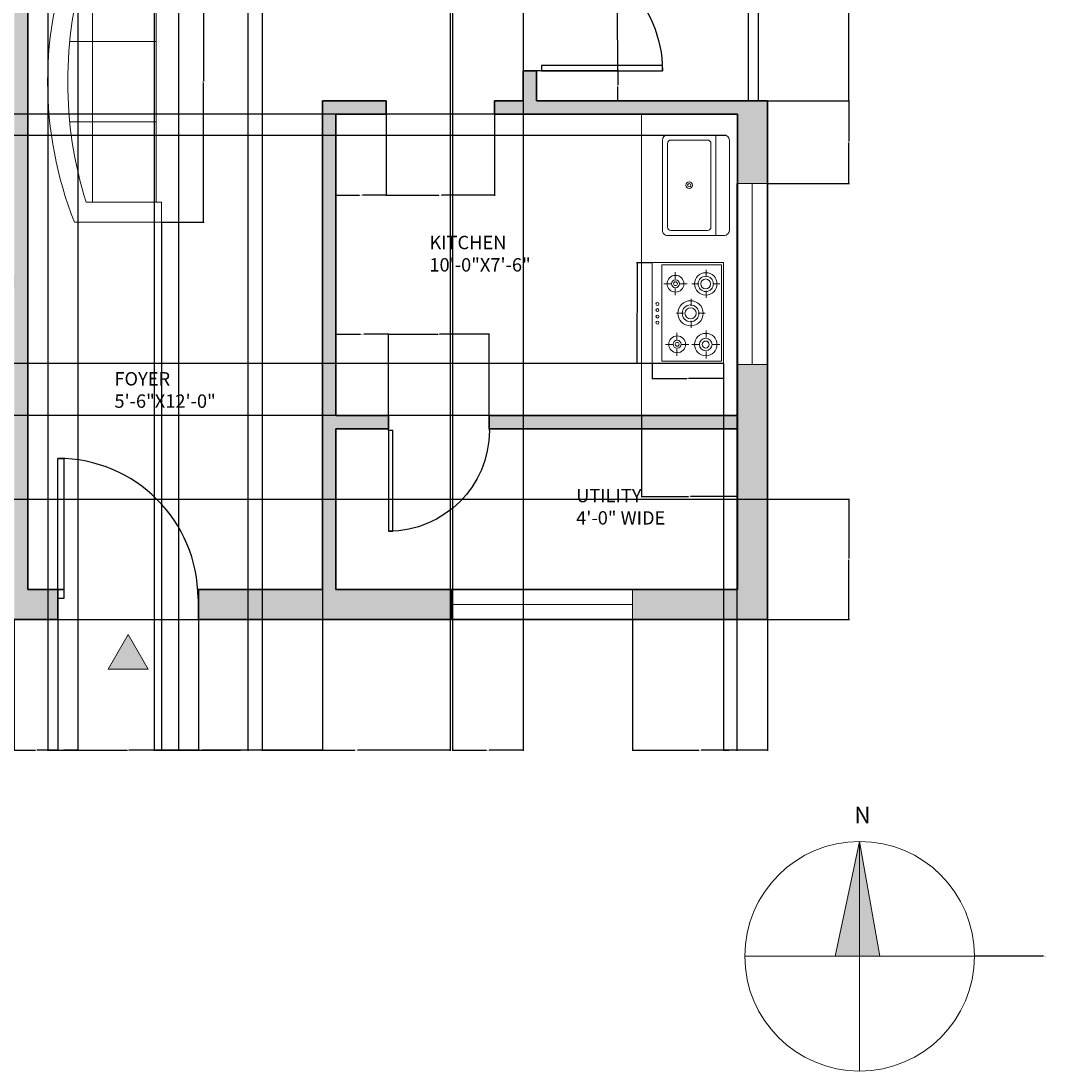
# Model space of a CAD drawing. Units: inches. Extents: x -29 to 443, y -589 to 39.
# Tile 2 of 5: x 136 to 443, y -589 to -275. Entities that reach past the tile are written whole.
import ezdxf

# ---------------------------------------------------------------- set-up
doc = ezdxf.new("R2010")
doc.units = ezdxf.units.IN
for name, color, linetype, lineweight in [('A-ANNO-DIMS', 2, 'Continuous', 18), ('A-ANNO-SYMB', 7, 'Continuous', 18), ('A-AREA-IDEN', 7, 'Continuous', 18), ('A-DOOR', 3, 'Continuous', 25), ('A-EQPM', 8, 'Continuous', 18), ('A-FLOR-CASE', 8, 'Continuous', 18), ('A-FLOR-FIXT', 9, 'Continuous', 18), ('A-FLOR-HRAL', 8, 'Continuous', 25), ('A-FURN', 9, 'Continuous', 18), ('A-GLAZ', 4, 'Continuous', 18), ('A-WALL', 7, 'Continuous', 35)]:
    doc.layers.add(name, color=color, linetype=linetype, lineweight=lineweight)
doc.layers.add('A-WALL-PATT', color=251, linetype='Continuous', lineweight=13, true_color=0x636466)
doc.styles.get("Standard").update_dxf_attribs({"font": 'arial.ttf'})
doc.dimstyles.get("Standard").update_dxf_attribs({"dimtxt": 0.18, "dimasz": 0.18, "dimexe": 0.18, "dimexo": 0.0625, "dimgap": 0.09, "dimtad": 0, "dimtih": 1, "dimtoh": 1, "dimdec": 4, "dimzin": 0, "dimdsep": 46, "dimtxsty": 'Standard', "dimcen": 0.09, "dimadec": 0, "dimazin": 0, "dimtfac": 1, "dimtdec": 4, "dimtofl": 0, "dimtmove": 0, "dimatfit": 3, "dimfxl": 1, "dimtolj": 1, "dimtzin": 0, "dimarcsym": 0})

# ---------------------------------------------------------------- blocks, each defined once
blk = doc.blocks.new('*U3')
for p, q in [((0, 0), (0, -6)), ((40, 0), (40, -6))]:
    blk.add_line(p, q)
blk.add_lwpolyline([(0, 0), (0, 40), (1.75, 40), (1.75, 0)], close=True)
blk.add_arc((0, 0), 40, 0, 90)
blk = doc.blocks.new('Sofa - Roundback 7 ft.')
for p, q in [((-12.00002, -32.4421), (-12.00003, -6.5971)), ((11.99997, -32.4421), (11.99998, -6.5971)), ((-36.000027, -34), (-36.000027, -11.4696)), ((35.99998, -34), (35.99998, -11.4696)), ((-35.999844, -13.3819), (35.9998, -13.3819)), ((-36.000027, -32.4421), (35.99998, -32.4421))]:
    blk.add_line(p, q)
for points in [[(-36.000027, -34), (-42.000027, -34), (-42.000027, -8)], [(41.99998, -8), (41.99998, -34), (35.99998, -34)]]:
    blk.add_lwpolyline(points)
for centre, radius, start, end in [((0, -114.25), 114.25, 68.43141, 111.5686), ((-0.00001, -127.1968), 121.1968, 72.72033, 107.2797)]:
    blk.add_arc(centre, radius, start, end)
blk = doc.blocks.new('Sink-single - 30 in top')
blk.add_line((-15, -3.999996), (15, -3.999996))
for points in [[(-13.5, 0), (13.5, 0)], [(-15, -18.499996), (-15, -1.5)], [(15, -1.5), (15, -18.499996)], [(-12.5, -5.499996), (12.5, -5.499996)], [(-13.5, -17.499996), (-13.5, -6.499996)], [(13.5, -6.499996), (13.5, -17.499996)], [(12.5, -18.499996), (-12.5, -18.499996)], [(13.5, -19.999996), (-13.5, -19.999996)]]:
    blk.add_lwpolyline(points)
for radius in [1, 0.5]:
    blk.add_circle((0, -11.999996), radius)
for centre, radius, start, end in [((-13.5, -1.5), 1.5, 90, 180), ((13.5, -1.5), 1.5, 0, 90), ((-12.5, -6.499996), 1, 90, 180), ((12.5, -6.499996), 1, 0, 90), ((-13.5, -18.499996), 1.5, 180, 270), ((-12.5, -17.499996), 1, 180, 270), ((12.5, -17.499996), 1, 270, 0), ((13.5, -18.499996), 1.5, 270, 0)]:
    blk.add_arc(centre, radius, start, end)
blk = doc.blocks.new('38')
at = {"color": 0}
for p, q in [((4682.26, 13565.85), (4682.26, 13514.85)), ((4754.26, 13565.85), (4682.26, 13565.85)), ((4683.76, 13564.35), (4683.76, 13521.85)), ((4752.76, 13564.35), (4683.76, 13564.35)), ((4697.41, 13558.27), (4697.41, 13563.27)), ((4740.78, 13558.27), (4740.78, 13563.27)), ((4752.76, 13521.85), (4752.76, 13564.35)), ((4754.26, 13514.85), (4754.26, 13565.85)), ((4692.48, 13553.34), (4687.47, 13553.34)), ((4697.41, 13543.15), (4697.41, 13548.16)), ((4707.33, 13553.34), (4702.32, 13553.34)), ((4718.43, 13547.65), (4718.43, 13552.65)), ((4735.85, 13553.34), (4730.84, 13553.34)), ((4740.78, 13543.15), (4740.78, 13548.16)), ((4750.7, 13553.34), (4745.7, 13553.34)), ((4697.4, 13534.82), (4697.4, 13539.82)), ((4713.11, 13542.65), (4708.11, 13542.65)), ((4728.85, 13542.65), (4723.85, 13542.65)), ((4740.72, 13536), (4740.72, 13541.01)), ((4718.43, 13532.28), (4718.43, 13537.28)), ((4737.37, 13532.58), (4732.37, 13532.58)), ((4748.92, 13532.58), (4743.92, 13532.58)), ((4694.05, 13531.4), (4689.04, 13531.4)), ((4697.45, 13523.21), (4697.45, 13528.21)), ((4705.6, 13531.4), (4700.6, 13531.4)), ((4740.78, 13524.39), (4740.78, 13529.4)), ((4683.76, 13521.85), (4752.76, 13521.85)), ((4682.26, 13514.85), (4754.26, 13514.85))]:
    blk.add_line(p, q, dxfattribs=at)
for centre, radius in [((4697.43, 13553.15), 8), ((4697.43, 13553.15), 5.5), ((4697.43, 13553.15), 3.5), ((4740.8, 13553.15), 8), ((4740.8, 13553.15), 4.5), ((4740.8, 13553.15), 2.5), ((4718.49, 13542.29), 9), ((4718.49, 13542.29), 6), ((4718.49, 13542.29), 4), ((4697.32, 13531.51), 6), ((4697.32, 13531.51), 2.85), ((4697.32, 13531.51), 1.35), ((4740.65, 13532.69), 6), ((4740.65, 13532.69), 2.85), ((4740.65, 13532.69), 1.35), ((4711.82, 13518.62), 1.09), ((4716.19, 13518.62), 1.09), ((4720.78, 13518.62), 1.09), ((4725.16, 13518.62), 1.09)]:
    blk.add_circle(centre, radius, dxfattribs=at)
blk = doc.blocks.new('WIN-54IN')
blk.add_line((54, 4.5), (0, 4.5))
blk.add_lwpolyline([(0, 9), (54, 9), (54, 0), (0, 0)], close=True)
blk = doc.blocks.new('*D30')
at = {"layer": 'A-ANNO-DIMS', "color": 0, "lineweight": -2, "transparency": 16777216}
for p, q in [((178.45, -250.92), (191.17, -250.92)), ((190.99, -251.1), (190.99, -292.74)), ((190.99, -334.74), (190.99, -293.11)), ((178.45, -334.92), (191.17, -334.92))]:
    blk.add_line(p, q, dxfattribs=at)
at = {"layer": 'A-ANNO-DIMS', "color": 0, "transparency": 16777216}
for points in [[(190.96, -251.1), (191.02, -251.1), (190.99, -250.92)], [(190.96, -334.74), (191.02, -334.74), (190.99, -334.92)]]:
    blk.add_solid(points, dxfattribs=at)
at = {"layer": 'Defpoints', "color": 0, "transparency": 16777216}
for p in [(178.39, -250.92), (190.99, -250.92), (178.39, -334.92)]:
    blk.add_point(p, dxfattribs=at)
at = {"layer": 'A-ANNO-DIMS', "color": 0, "transparency": 16777216, "insert": (190.99, -292.92), "char_height": 0.18, "attachment_point": 5}
blk.add_mtext('\\A1;SOFA 84', dxfattribs=at)
blk = doc.blocks.new('*D34')
at = {"layer": 'A-ANNO-DIMS', "color": 0, "lineweight": -2, "transparency": 16777216}
for p, q in [((324.89, -346.99), (320.26, -346.99)), ((320.44, -347.17), (320.44, -361.85)), ((320.44, -376.89), (320.44, -362.21)), ((324.89, -377.07), (320.26, -377.07))]:
    blk.add_line(p, q, dxfattribs=at)
at = {"layer": 'A-ANNO-DIMS', "color": 0, "transparency": 16777216}
for points in [[(320.41, -347.17), (320.47, -347.17), (320.44, -346.99)], [(320.41, -376.89), (320.47, -376.89), (320.44, -377.07)]]:
    blk.add_solid(points, dxfattribs=at)
at = {"layer": 'Defpoints', "color": 0, "transparency": 16777216}
for p in [(324.95, -346.99), (320.44, -377.07), (324.95, -377.07)]:
    blk.add_point(p, dxfattribs=at)
at = {"layer": 'A-ANNO-DIMS', "color": 0, "transparency": 16777216, "insert": (320.44, -362.03), "char_height": 0.18, "attachment_point": 5}
blk.add_mtext('\\A1;COOKTOP 30', dxfattribs=at)
blk = doc.blocks.new('*D35')
at = {"layer": 'A-ANNO-DIMS', "color": 0, "lineweight": -2, "transparency": 16777216}
for p, q in [((324.95, -377.13), (324.95, -381.76)), ((346.26, -377.13), (346.26, -381.76)), ((325.13, -381.58), (335.41, -381.58)), ((346.08, -381.58), (335.81, -381.58))]:
    blk.add_line(p, q, dxfattribs=at)
at = {"layer": 'A-ANNO-DIMS', "color": 0, "transparency": 16777216}
for points in [[(325.13, -381.55), (325.13, -381.61), (324.95, -381.58)], [(346.08, -381.55), (346.08, -381.61), (346.26, -381.58)]]:
    blk.add_solid(points, dxfattribs=at)
at = {"layer": 'Defpoints', "color": 0, "transparency": 16777216}
for p in [(324.95, -377.07), (346.26, -377.07), (346.26, -381.58)]:
    blk.add_point(p, dxfattribs=at)
at = {"layer": 'A-ANNO-DIMS', "color": 0, "transparency": 16777216, "insert": (335.61, -381.58), "char_height": 0.18, "attachment_point": 5}
blk.add_mtext('\\A1;21', dxfattribs=at)
blk = doc.blocks.new('*D40')
at = {"layer": 'A-ANNO-DIMS', "color": 0, "lineweight": -2, "transparency": 16777216}
for p, q in [((208.44, 5.32), (208.44, -492.89)), ((264.58, 5.32), (264.58, -492.89)), ((208.62, -492.71), (236.11, -492.71)), ((264.4, -492.71), (236.9, -492.71))]:
    blk.add_line(p, q, dxfattribs=at)
at = {"layer": 'A-ANNO-DIMS', "color": 0, "transparency": 16777216}
for points in [[(208.62, -492.68), (208.62, -492.74), (208.44, -492.71)], [(264.4, -492.68), (264.4, -492.74), (264.58, -492.71)]]:
    blk.add_solid(points, dxfattribs=at)
at = {"layer": 'Defpoints', "color": 0, "transparency": 16777216}
for p in [(208.44, 5.39), (264.58, 5.39), (208.44, -492.71)]:
    blk.add_point(p, dxfattribs=at)
at = {"layer": 'A-ANNO-DIMS', "color": 0, "transparency": 16777216, "insert": (236.51, -492.71), "char_height": 0.18, "attachment_point": 5}
blk.add_mtext('\\A1;56.14', dxfattribs=at)
blk = doc.blocks.new('*D42')
at = {"layer": 'A-ANNO-DIMS', "color": 0, "lineweight": -2, "transparency": 16777216}
for p, q in [((114.5, -417.61), (383.85, -417.61)), ((383.67, -417.79), (383.67, -435.43)), ((383.67, -453.43), (383.67, -435.8)), ((134.5, -453.61), (383.85, -453.61))]:
    blk.add_line(p, q, dxfattribs=at)
at = {"layer": 'A-ANNO-DIMS', "color": 0, "transparency": 16777216}
for points in [[(383.64, -417.79), (383.7, -417.79), (383.67, -417.61)], [(383.64, -453.43), (383.7, -453.43), (383.67, -453.61)]]:
    blk.add_solid(points, dxfattribs=at)
at = {"layer": 'Defpoints', "color": 0, "transparency": 16777216}
for p in [(114.44, -417.61), (134.44, -453.61), (383.67, -453.61)]:
    blk.add_point(p, dxfattribs=at)
at = {"layer": 'A-ANNO-DIMS', "color": 0, "transparency": 16777216, "insert": (383.67, -435.61), "char_height": 0.18, "attachment_point": 5}
blk.add_mtext('\\A1;36', dxfattribs=at)
blk = doc.blocks.new('*D43')
at = {"layer": 'A-ANNO-DIMS', "color": 0, "lineweight": -2, "transparency": 16777216}
for p, q in [((359.5, -298.61), (383.85, -298.61)), ((383.67, -298.79), (383.67, -310.81)), ((383.67, -323.2), (383.67, -311.18)), ((359.33, -323.38), (383.85, -323.38))]:
    blk.add_line(p, q, dxfattribs=at)
at = {"layer": 'A-ANNO-DIMS', "color": 0, "transparency": 16777216}
for points in [[(383.64, -298.79), (383.7, -298.79), (383.67, -298.61)], [(383.64, -323.2), (383.7, -323.2), (383.67, -323.38)]]:
    blk.add_solid(points, dxfattribs=at)
at = {"layer": 'Defpoints', "color": 0, "transparency": 16777216}
for p in [(359.44, -298.61), (383.67, -298.61), (359.27, -323.38)]:
    blk.add_point(p, dxfattribs=at)
at = {"layer": 'A-ANNO-DIMS', "color": 0, "transparency": 16777216, "insert": (383.67, -311), "char_height": 0.18, "attachment_point": 5}
blk.add_mtext('\\A1;24.76', dxfattribs=at)
blk = doc.blocks.new('*D45')
at = {"layer": 'A-ANNO-DIMS', "color": 0, "lineweight": -2, "transparency": 16777216}
for p, q in [((359.5, -154.61), (383.85, -154.61)), ((383.67, -154.79), (383.67, -226.43)), ((383.67, -298.43), (383.67, -226.8)), ((359.5, -298.61), (383.85, -298.61))]:
    blk.add_line(p, q, dxfattribs=at)
at = {"layer": 'A-ANNO-DIMS', "color": 0, "transparency": 16777216}
for points in [[(383.64, -154.79), (383.7, -154.79), (383.67, -154.61)], [(383.64, -298.43), (383.7, -298.43), (383.67, -298.61)]]:
    blk.add_solid(points, dxfattribs=at)
at = {"layer": 'Defpoints', "color": 0, "transparency": 16777216}
for p in [(359.44, -154.61), (359.44, -298.61), (383.67, -298.61)]:
    blk.add_point(p, dxfattribs=at)
at = {"layer": 'A-ANNO-DIMS', "color": 0, "transparency": 16777216, "insert": (383.67, -226.61), "char_height": 0.18, "attachment_point": 5}
blk.add_mtext('\\A1;144', dxfattribs=at)
blk = doc.blocks.new('*D49')
at = {"layer": 'A-ANNO-DIMS', "color": 0, "lineweight": -2, "transparency": 16777216}
for p, q in [((319.03, -453.7), (319.03, -492.89)), ((359.44, -453.68), (359.44, -492.89)), ((319.21, -492.71), (338.85, -492.71)), ((359.26, -492.71), (339.61, -492.71))]:
    blk.add_line(p, q, dxfattribs=at)
at = {"layer": 'A-ANNO-DIMS', "color": 0, "transparency": 16777216}
for points in [[(319.21, -492.68), (319.21, -492.74), (319.03, -492.71)], [(359.26, -492.68), (359.26, -492.74), (359.44, -492.71)]]:
    blk.add_solid(points, dxfattribs=at)
at = {"layer": 'Defpoints', "color": 0, "transparency": 16777216}
for p in [(319.03, -453.64), (359.44, -453.61), (359.44, -492.71)]:
    blk.add_point(p, dxfattribs=at)
at = {"layer": 'A-ANNO-DIMS', "color": 0, "transparency": 16777216, "insert": (339.23, -492.71), "char_height": 0.18, "attachment_point": 5}
blk.add_mtext('\\A1;40.41', dxfattribs=at)
blk = doc.blocks.new('*D52')
at = {"layer": 'A-ANNO-DIMS', "color": 0, "lineweight": -2, "transparency": 16777216}
for p, q in [((153.44, -94.68), (153.44, -492.89)), ((183.44, -94.68), (183.44, -492.89)), ((153.62, -492.71), (168.22, -492.71)), ((183.26, -492.71), (168.65, -492.71))]:
    blk.add_line(p, q, dxfattribs=at)
at = {"layer": 'A-ANNO-DIMS', "color": 0, "transparency": 16777216}
for points in [[(153.62, -492.68), (153.62, -492.74), (153.44, -492.71)], [(183.26, -492.68), (183.26, -492.74), (183.44, -492.71)]]:
    blk.add_solid(points, dxfattribs=at)
at = {"layer": 'Defpoints', "color": 0, "transparency": 16777216}
for p in [(153.44, -94.61), (183.44, -94.61), (183.44, -492.71)]:
    blk.add_point(p, dxfattribs=at)
at = {"layer": 'A-ANNO-DIMS', "color": 0, "transparency": 16777216, "insert": (168.44, -492.71), "char_height": 0.18, "attachment_point": 5}
blk.add_mtext('\\A1;30', dxfattribs=at)
blk = doc.blocks.new('*D53')
at = {"layer": 'A-ANNO-DIMS', "color": 0, "lineweight": -2, "transparency": 16777216}
for p, q in [((147.44, -453.68), (147.44, -492.89)), ((189.44, -453.68), (189.44, -492.89)), ((147.62, -492.71), (168.21, -492.71)), ((189.26, -492.71), (168.66, -492.71))]:
    blk.add_line(p, q, dxfattribs=at)
at = {"layer": 'A-ANNO-DIMS', "color": 0, "transparency": 16777216}
for points in [[(147.62, -492.68), (147.62, -492.74), (147.44, -492.71)], [(189.26, -492.68), (189.26, -492.74), (189.44, -492.71)]]:
    blk.add_solid(points, dxfattribs=at)
at = {"layer": 'Defpoints', "color": 0, "transparency": 16777216}
for p in [(147.44, -453.61), (189.44, -453.61), (189.44, -492.71)]:
    blk.add_point(p, dxfattribs=at)
at = {"layer": 'A-ANNO-DIMS', "color": 0, "transparency": 16777216, "insert": (168.44, -492.71), "char_height": 0.18, "attachment_point": 5}
blk.add_mtext('\\A1;42', dxfattribs=at)
blk = doc.blocks.new('*D54')
at = {"layer": 'A-ANNO-DIMS', "color": 0, "lineweight": -2, "transparency": 16777216}
for p, q in [((134.44, -453.68), (134.44, -492.89)), ((147.44, -453.68), (147.44, -492.89)), ((134.62, -492.71), (140.73, -492.71)), ((147.26, -492.71), (141.15, -492.71))]:
    blk.add_line(p, q, dxfattribs=at)
at = {"layer": 'A-ANNO-DIMS', "color": 0, "transparency": 16777216}
for points in [[(134.62, -492.68), (134.62, -492.74), (134.44, -492.71)], [(147.26, -492.68), (147.26, -492.74), (147.44, -492.71)]]:
    blk.add_solid(points, dxfattribs=at)
at = {"layer": 'Defpoints', "color": 0, "transparency": 16777216}
for p in [(134.44, -453.61), (147.44, -453.61), (147.44, -492.71)]:
    blk.add_point(p, dxfattribs=at)
at = {"layer": 'A-ANNO-DIMS', "color": 0, "transparency": 16777216, "insert": (140.94, -492.71), "char_height": 0.18, "attachment_point": 5}
blk.add_mtext('\\A1;13', dxfattribs=at)
blk = doc.blocks.new('*D55')
at = {"layer": 'A-ANNO-DIMS', "color": 0, "lineweight": -2, "transparency": 16777216}
for p, q in [((290.34, -253.47), (314.69, -253.36)), ((314.51, -253.54), (314.59, -271.25)), ((314.66, -289.33), (314.59, -271.62)), ((290.5, -289.61), (314.85, -289.51))]:
    blk.add_line(p, q, dxfattribs=at)
at = {"layer": 'A-ANNO-DIMS', "color": 0, "transparency": 16777216}
for points in [[(314.54, -253.54), (314.48, -253.54), (314.51, -253.36)], [(314.69, -289.33), (314.63, -289.33), (314.67, -289.51)]]:
    blk.add_solid(points, dxfattribs=at)
at = {"layer": 'Defpoints', "color": 0, "transparency": 16777216}
for p in [(290.28, -253.47), (290.44, -289.61), (314.67, -289.51)]:
    blk.add_point(p, dxfattribs=at)
at = {"layer": 'A-ANNO-DIMS', "color": 0, "transparency": 16777216, "insert": (314.59, -271.44), "char_height": 0.18, "attachment_point": 5}
blk.add_mtext('\\A1;36.15', dxfattribs=at)
blk = doc.blocks.new('*D56')
at = {"layer": 'A-ANNO-DIMS', "color": 0, "lineweight": -2, "transparency": 16777216}
for p, q in [((290.5, -289.61), (314.85, -289.61)), ((314.67, -289.79), (314.67, -293.93)), ((314.67, -298.43), (314.67, -294.3)), ((290.5, -298.61), (314.85, -298.61))]:
    blk.add_line(p, q, dxfattribs=at)
at = {"layer": 'A-ANNO-DIMS', "color": 0, "transparency": 16777216}
for points in [[(314.64, -289.79), (314.7, -289.79), (314.67, -289.61)], [(314.64, -298.43), (314.7, -298.43), (314.67, -298.61)]]:
    blk.add_solid(points, dxfattribs=at)
at = {"layer": 'Defpoints', "color": 0, "transparency": 16777216}
for p in [(290.44, -289.61), (290.44, -298.61), (314.67, -298.61)]:
    blk.add_point(p, dxfattribs=at)
at = {"layer": 'A-ANNO-DIMS', "color": 0, "transparency": 16777216, "insert": (314.67, -294.11), "char_height": 0.18, "attachment_point": 5}
blk.add_mtext('\\A1;9', dxfattribs=at)
blk = doc.blocks.new('*D57')
at = {"layer": 'A-ANNO-DIMS', "color": 0, "lineweight": -2, "transparency": 16777216}
for p, q in [((246.22, -392.55), (246.22, -368.2)), ((246.4, -368.38), (261, -368.38)), ((276.04, -368.38), (261.44, -368.38)), ((276.22, -392.55), (276.22, -368.2))]:
    blk.add_line(p, q, dxfattribs=at)
at = {"layer": 'A-ANNO-DIMS', "color": 0, "transparency": 16777216}
for points in [[(246.4, -368.35), (246.4, -368.41), (246.22, -368.38)], [(276.04, -368.35), (276.04, -368.41), (276.22, -368.38)]]:
    blk.add_solid(points, dxfattribs=at)
at = {"layer": 'Defpoints', "color": 0, "transparency": 16777216}
for p in [(276.22, -368.38), (246.22, -392.61), (276.22, -392.61)]:
    blk.add_point(p, dxfattribs=at)
at = {"layer": 'A-ANNO-DIMS', "color": 0, "transparency": 16777216, "insert": (261.22, -368.38), "char_height": 0.18, "attachment_point": 5}
blk.add_mtext('\\A1;30', dxfattribs=at)
blk = doc.blocks.new('*D58')
at = {"layer": 'A-ANNO-DIMS', "color": 0, "lineweight": -2, "transparency": 16777216}
for p, q in [((230.44, -392.55), (230.44, -368.2)), ((230.62, -368.38), (237.87, -368.38)), ((246.04, -368.38), (238.78, -368.38)), ((246.22, -392.55), (246.22, -368.2))]:
    blk.add_line(p, q, dxfattribs=at)
at = {"layer": 'A-ANNO-DIMS', "color": 0, "transparency": 16777216}
for points in [[(230.62, -368.35), (230.62, -368.41), (230.44, -368.38)], [(246.04, -368.35), (246.04, -368.41), (246.22, -368.38)]]:
    blk.add_solid(points, dxfattribs=at)
at = {"layer": 'Defpoints', "color": 0, "transparency": 16777216}
for p in [(246.22, -368.38), (230.44, -392.61), (246.22, -392.61)]:
    blk.add_point(p, dxfattribs=at)
at = {"layer": 'A-ANNO-DIMS', "color": 0, "transparency": 16777216, "insert": (238.33, -368.38), "char_height": 0.18, "attachment_point": 5}
blk.add_mtext('\\A1;15.787', dxfattribs=at)
blk = doc.blocks.new('*D60')
at = {"layer": 'A-ANNO-DIMS', "color": 0, "lineweight": -2, "transparency": 16777216}
for p, q in [((245.49, -302.68), (245.49, -327.02)), ((277.84, -302.68), (277.84, -327.02)), ((245.67, -326.84), (261.27, -326.84)), ((277.66, -326.84), (262.06, -326.84))]:
    blk.add_line(p, q, dxfattribs=at)
at = {"layer": 'A-ANNO-DIMS', "color": 0, "transparency": 16777216}
for points in [[(245.67, -326.81), (245.67, -326.87), (245.49, -326.84)], [(277.66, -326.81), (277.66, -326.87), (277.84, -326.84)]]:
    blk.add_solid(points, dxfattribs=at)
at = {"layer": 'Defpoints', "color": 0, "transparency": 16777216}
for p in [(245.49, -302.61), (277.84, -302.61), (245.49, -326.84)]:
    blk.add_point(p, dxfattribs=at)
at = {"layer": 'A-ANNO-DIMS', "color": 0, "transparency": 16777216, "insert": (261.66, -326.84), "char_height": 0.18, "attachment_point": 5}
blk.add_mtext('\\A1;32.35', dxfattribs=at)
blk = doc.blocks.new('*D61')
at = {"layer": 'A-ANNO-DIMS', "color": 0, "lineweight": -2, "transparency": 16777216}
for p, q in [((230.44, -302.68), (230.44, -327.02)), ((245.49, -302.68), (245.49, -327.02)), ((230.62, -326.84), (237.51, -326.84)), ((245.31, -326.84), (238.42, -326.84))]:
    blk.add_line(p, q, dxfattribs=at)
at = {"layer": 'A-ANNO-DIMS', "color": 0, "transparency": 16777216}
for points in [[(230.62, -326.81), (230.62, -326.87), (230.44, -326.84)], [(245.31, -326.81), (245.31, -326.87), (245.49, -326.84)]]:
    blk.add_solid(points, dxfattribs=at)
at = {"layer": 'Defpoints', "color": 0, "transparency": 16777216}
for p in [(230.44, -302.61), (245.49, -302.61), (230.44, -326.84)]:
    blk.add_point(p, dxfattribs=at)
at = {"layer": 'A-ANNO-DIMS', "color": 0, "transparency": 16777216, "insert": (237.96, -326.84), "char_height": 0.18, "attachment_point": 5}
blk.add_mtext('\\A1;15.053', dxfattribs=at)
blk = doc.blocks.new('*D68')
at = {"layer": 'A-ANNO-DIMS', "color": 0, "lineweight": -2, "transparency": 16777216}
for p, q in [((176.21, -22.71), (176.21, -492.89)), ((204.21, -33.21), (204.21, -492.89)), ((176.39, -492.71), (189.99, -492.71)), ((204.03, -492.71), (190.43, -492.71))]:
    blk.add_line(p, q, dxfattribs=at)
at = {"layer": 'A-ANNO-DIMS', "color": 0, "transparency": 16777216}
for points in [[(176.39, -492.68), (176.39, -492.74), (176.21, -492.71)], [(204.03, -492.68), (204.03, -492.74), (204.21, -492.71)]]:
    blk.add_solid(points, dxfattribs=at)
at = {"layer": 'Defpoints', "color": 0, "transparency": 16777216}
for p in [(176.21, -22.65), (204.21, -33.15), (204.21, -492.71)]:
    blk.add_point(p, dxfattribs=at)
at = {"layer": 'A-ANNO-DIMS', "color": 0, "transparency": 16777216, "insert": (190.21, -492.71), "char_height": 0.18, "attachment_point": 5}
blk.add_mtext('\\A1;28', dxfattribs=at)
blk = doc.blocks.new('*D71')
at = {"layer": 'A-ANNO-DIMS', "color": 0, "lineweight": -2, "transparency": 16777216}
for p, q in [((144.44, -94.68), (144.44, -492.89)), ((153.44, -94.68), (153.44, -492.89)), ((144.62, -492.71), (148.79, -492.71)), ((153.26, -492.71), (149.09, -492.71))]:
    blk.add_line(p, q, dxfattribs=at)
at = {"layer": 'A-ANNO-DIMS', "color": 0, "transparency": 16777216}
for points in [[(144.62, -492.68), (144.62, -492.74), (144.44, -492.71)], [(153.26, -492.68), (153.26, -492.74), (153.44, -492.71)]]:
    blk.add_solid(points, dxfattribs=at)
at = {"layer": 'Defpoints', "color": 0, "transparency": 16777216}
for p in [(144.44, -94.61), (153.44, -94.61), (153.44, -492.71)]:
    blk.add_point(p, dxfattribs=at)
at = {"layer": 'A-ANNO-DIMS', "color": 0, "transparency": 16777216, "insert": (148.94, -492.71), "char_height": 0.18, "attachment_point": 5}
blk.add_mtext('\\A1;9', dxfattribs=at)
blk = doc.blocks.new('*D73')
at = {"layer": 'A-ANNO-DIMS', "color": 0, "lineweight": -2, "transparency": 16777216}
for p, q in [((321.74, -392.68), (321.74, -417.02)), ((350.44, -392.68), (350.44, -417.02)), ((321.92, -416.84), (335.76, -416.84)), ((350.26, -416.84), (336.41, -416.84))]:
    blk.add_line(p, q, dxfattribs=at)
at = {"layer": 'A-ANNO-DIMS', "color": 0, "transparency": 16777216}
for points in [[(321.92, -416.81), (321.92, -416.87), (321.74, -416.84)], [(350.26, -416.81), (350.26, -416.87), (350.44, -416.84)]]:
    blk.add_solid(points, dxfattribs=at)
at = {"layer": 'Defpoints', "color": 0, "transparency": 16777216}
for p in [(321.74, -392.61), (350.44, -392.61), (321.74, -416.84)]:
    blk.add_point(p, dxfattribs=at)
at = {"layer": 'A-ANNO-DIMS', "color": 0, "transparency": 16777216, "insert": (336.09, -416.84), "char_height": 0.18, "attachment_point": 5}
blk.add_mtext('\\A1;28.7', dxfattribs=at)
blk = doc.blocks.new('*D74')
at = {"layer": 'A-ANNO-DIMS', "color": 0, "lineweight": -2, "transparency": 16777216}
for p, q in [((286.44, -169.54), (286.44, -492.89)), ((265.28, -188.07), (265.28, -492.89)), ((265.46, -492.71), (275.46, -492.71)), ((286.26, -492.71), (276.26, -492.71))]:
    blk.add_line(p, q, dxfattribs=at)
at = {"layer": 'A-ANNO-DIMS', "color": 0, "transparency": 16777216}
for points in [[(265.46, -492.68), (265.46, -492.74), (265.28, -492.71)], [(286.26, -492.68), (286.26, -492.74), (286.44, -492.71)]]:
    blk.add_solid(points, dxfattribs=at)
at = {"layer": 'Defpoints', "color": 0, "transparency": 16777216}
for p in [(286.44, -169.48), (265.28, -188), (286.44, -492.71)]:
    blk.add_point(p, dxfattribs=at)
at = {"layer": 'A-ANNO-DIMS', "color": 0, "transparency": 16777216, "insert": (275.86, -492.71), "char_height": 0.18, "attachment_point": 5}
blk.add_mtext('\\A1;21.15', dxfattribs=at)
blk = doc.blocks.new('*D76')
at = {"layer": 'A-ANNO-DIMS', "color": 0, "lineweight": -2, "transparency": 16777216}
for p, q in [((346.26, -377.13), (346.26, -492.89)), ((350.27, -377.44), (350.27, -492.89)), ((346.44, -492.71), (347.87, -492.71)), ((350.09, -492.71), (348.66, -492.71))]:
    blk.add_line(p, q, dxfattribs=at)
at = {"layer": 'A-ANNO-DIMS', "color": 0, "transparency": 16777216}
for points in [[(346.44, -492.68), (346.44, -492.74), (346.26, -492.71)], [(350.09, -492.68), (350.09, -492.74), (350.27, -492.71)]]:
    blk.add_solid(points, dxfattribs=at)
at = {"layer": 'Defpoints', "color": 0, "transparency": 16777216}
for p in [(346.26, -377.07), (350.27, -377.38), (346.26, -492.71)]:
    blk.add_point(p, dxfattribs=at)
at = {"layer": 'A-ANNO-DIMS', "color": 0, "transparency": 16777216, "insert": (348.26, -492.71), "char_height": 0.18, "attachment_point": 5}
blk.add_mtext('\\A1;4.004', dxfattribs=at)
blk = doc.blocks.new('*D83')
at = {"layer": 'A-ANNO-DIMS', "color": 0, "lineweight": -2, "transparency": 16777216}
for p, q in [((226.44, -298.68), (226.44, -492.89)), ((178.39, -334.99), (178.39, -492.89)), ((178.57, -492.71), (202.02, -492.71)), ((226.26, -492.71), (202.81, -492.71))]:
    blk.add_line(p, q, dxfattribs=at)
at = {"layer": 'A-ANNO-DIMS', "color": 0, "transparency": 16777216}
for points in [[(178.57, -492.68), (178.57, -492.74), (178.39, -492.71)], [(226.26, -492.68), (226.26, -492.74), (226.44, -492.71)]]:
    blk.add_solid(points, dxfattribs=at)
at = {"layer": 'Defpoints', "color": 0, "transparency": 16777216}
for p in [(226.44, -298.61), (178.39, -334.92), (226.44, -492.71)]:
    blk.add_point(p, dxfattribs=at)
at = {"layer": 'A-ANNO-DIMS', "color": 0, "transparency": 16777216, "insert": (202.41, -492.71), "char_height": 0.18, "attachment_point": 5}
blk.add_mtext('\\A1;48.05', dxfattribs=at)
blk = doc.blocks.new('*D84')
at = {"layer": 'A-ANNO-DIMS', "color": 0, "lineweight": -2, "transparency": 16777216}
for p, q in [((350.37, -302.61), (-28.85, -302.61)), ((-28.67, -302.79), (-28.67, -305.61)), ((-28.67, -308.79), (-28.67, -305.97)), ((347.03, -308.97), (-28.85, -308.97))]:
    blk.add_line(p, q, dxfattribs=at)
at = {"layer": 'A-ANNO-DIMS', "color": 0, "transparency": 16777216}
for points in [[(-28.7, -302.79), (-28.64, -302.79), (-28.67, -302.61)], [(-28.7, -308.79), (-28.64, -308.79), (-28.67, -308.97)]]:
    blk.add_solid(points, dxfattribs=at)
at = {"layer": 'Defpoints', "color": 0, "transparency": 16777216}
for p in [(350.44, -302.61), (-28.67, -308.97), (347.09, -308.97)]:
    blk.add_point(p, dxfattribs=at)
at = {"layer": 'A-ANNO-DIMS', "color": 0, "transparency": 16777216, "insert": (-28.67, -305.79), "char_height": 0.18, "attachment_point": 5}
blk.add_mtext('\\A1;6.353', dxfattribs=at)
blk = doc.blocks.new('*D85')
at = {"layer": 'A-ANNO-DIMS', "color": 0, "lineweight": -2, "transparency": 16777216}
for p, q in [((346.2, -377.07), (-28.85, -377.07)), ((-28.67, -377.25), (-28.67, -384.66)), ((-28.67, -392.43), (-28.67, -385.02)), ((350.37, -392.61), (-28.85, -392.61))]:
    blk.add_line(p, q, dxfattribs=at)
at = {"layer": 'A-ANNO-DIMS', "color": 0, "transparency": 16777216}
for points in [[(-28.7, -377.25), (-28.64, -377.25), (-28.67, -377.07)], [(-28.7, -392.43), (-28.64, -392.43), (-28.67, -392.61)]]:
    blk.add_solid(points, dxfattribs=at)
at = {"layer": 'Defpoints', "color": 0, "transparency": 16777216}
for p in [(-28.67, -377.07), (346.26, -377.07), (350.44, -392.61)]:
    blk.add_point(p, dxfattribs=at)
at = {"layer": 'A-ANNO-DIMS', "color": 0, "transparency": 16777216, "insert": (-28.67, -384.84), "char_height": 0.18, "attachment_point": 5}
blk.add_mtext('\\A1;15.544', dxfattribs=at)
blk = doc.blocks.new('*D86')
at = {"layer": 'A-ANNO-DIMS', "color": 0, "lineweight": -2, "transparency": 16777216}
for p, q in [((386.82, -554.23), (387, -554.23)), ((386.91, -554.32), (386.91, -554.14)), ((441.79, -554.24), (421.39, -554.24))]:
    blk.add_line(p, q, dxfattribs=at)
at = {"layer": 'A-ANNO-DIMS', "color": 0, "transparency": 16777216}
blk.add_solid([(421.39, -554.21), (421.39, -554.27), (421.21, -554.24)], dxfattribs=at)
at = {"layer": 'Defpoints', "color": 0, "transparency": 16777216}
for p in [(352.62, -554.23), (421.21, -554.24)]:
    blk.add_point(p, dxfattribs=at)
at = {"layer": 'A-ANNO-DIMS', "color": 0, "transparency": 16777216, "insert": (442.21, -554.24), "char_height": 0.18, "attachment_point": 5}
blk.add_mtext('\\A1;∅68.6', dxfattribs=at)

msp = doc.modelspace()

# ---------------------------------------------------------------- hatches: boundary and pattern name
at = {"layer": 'A-ANNO-SYMB'}
h = msp.add_hatch(color=256, dxfattribs=at)
h.dxf.hatch_style = 1
h.paths.add_polyline_path([(168.4202, -458.0922), (162.4202, -468.4845), (174.4202, -468.4845)])
h = msp.add_hatch(color=256, dxfattribs=at)
h.dxf.hatch_style = 1
h.paths.add_polyline_path([(386.9149, -519.9368), (379.5797, -554.2347), (386.9149, -554.2347)])
h.paths.add_polyline_path([(386.9149, -519.9368), (386.9149, -554.2347), (392.8984, -554.2347)])
at = {"layer": 'A-WALL-PATT'}
h = msp.add_hatch(color=256, dxfattribs=at)
h.dxf.hatch_style = 1
h.paths.add_polyline_path([(8.4359, 5.3851), (38.6638, 5.3851), (38.6638, 14.3851), (-0.5641, 14.3851), (-0.5641, -161.7206), (8.4359, -161.7206), (8.4359, -154.6149), (98.4359, -154.6149), (98.4359, -169.6149), (102.4359, -169.6149), (102.4359, -154.6149), (144.4359, -154.6149), (144.4359, -141.6149), (140.4359, -141.6149), (140.4359, -150.6149), (8.4359, -150.6149)])
h.paths.add_polyline_path([(153.762, 14.3851), (92.6638, 14.3851), (92.6638, 5.3851), (140.4359, 5.3851), (140.4359, -105.5868), (144.4359, -105.5868), (144.4359, -94.6149), (153.4359, -94.6149), (153.4359, -90.6149), (144.4359, -90.6149), (144.4359, 5.3851), (153.762, 5.3851)])
h.paths.add_polyline_path([(264.576, 14.3851), (189.762, 14.3851), (189.762, 5.3851), (204.4359, 5.3851), (204.4359, -40.0486, -0.11439146), (204.5889, -40.7086), (204.5889, -67.7086, -0.11439146), (204.4359, -68.3685), (204.4359, -90.6149), (183.4359, -90.6149), (183.4359, -94.6149), (204.4359, -94.6149), (204.4359, -108.4622), (208.4359, -108.4622), (208.4359, 5.3851), (264.576, 5.3851)])
h.paths.add_polyline_path([(359.4359, 14.3851), (318.576, 14.3851), (318.576, 5.3851), (350.4359, 5.3851), (350.4359, -150.6149), (208.4359, -150.6149), (208.4359, -144.6149), (204.4359, -144.6149), (204.4359, -154.6149), (286.4359, -154.6149), (286.4359, -169.4775), (290.4359, -169.4775), (290.4359, -154.6149), (359.4359, -154.6149)])
h.paths.add_polyline_path([(8.4359, -212.6149), (98.4359, -212.6149), (102.4359, -212.6149), (102.4359, -199.6149), (98.4359, -199.6149), (98.4359, -208.6149), (8.4359, -208.6149), (8.4359, -197.7206), (-0.5641, -197.7206), (-0.5641, -417.6149), (114.4359, -417.6149), (114.4359, -354.6149), (134.4359, -354.6149), (134.4359, -453.6149), (147.4359, -453.6149), (147.4359, -444.6149), (138.4359, -444.6149), (138.4359, -212.6149), (129.4359, -212.6149), (129.4359, -216.6149), (134.4359, -216.6149), (134.4359, -350.6149), (110.4359, -350.6149), (110.4359, -377.2063, -0.30395766), (111.1497, -378.2719, -0.30395766), (110.4359, -379.3376), (110.4359, -408.6149), (8.4359, -408.6149)])
h.paths.add_polyline_path([(265.0252, -444.6149), (230.4359, -444.6149), (230.4359, -396.6149), (246.223, -396.6149), (246.223, -392.6149), (230.4359, -392.6149), (230.4359, -302.6149), (245.4886, -302.6149), (245.4886, -298.6149), (226.4359, -298.6149), (226.4359, -444.6149), (189.4359, -444.6149), (189.4359, -453.6149), (226.4359, -453.6149), (265.0252, -453.6149)])
h.paths.add_polyline_path([(359.4359, -417.6149), (359.4359, -377.3771), (350.4359, -377.3771), (350.4359, -392.6149), (276.3235, -392.6149), (276.3235, -396.6149), (350.4359, -396.6149), (350.4359, -408.6149), (350.4359, -444.6149), (319.0252, -444.6149), (319.0252, -453.6149), (359.4359, -453.6149)])
h.paths.add_polyline_path([(359.4359, -298.6149), (290.4359, -298.6149), (290.4359, -289.6207), (286.4359, -289.6207), (286.4359, -298.6149), (277.8355, -298.6149), (277.8355, -302.6149), (350.4359, -302.6149), (350.4359, -323.3771), (359.4359, -323.3771)])
h.paths.add_polyline_path([(290.4359, -226.7916), (286.4359, -226.7916), (286.4359, -253.468), (290.4359, -253.468)])

# ---------------------------------------------------------------- linework, layer by layer
at = {"layer": 'A-ANNO-SYMB'}
for p, q in [((386.9149, -519.9368), (379.5797, -554.2347)), ((386.9149, -519.9368), (386.9149, -588.5325)), ((386.9149, -519.9368), (392.8984, -554.2347)), ((352.617, -554.2347), (421.2127, -554.2347))]:
    msp.add_line(p, q, dxfattribs=at)
msp.add_lwpolyline([(162.4202, -468.4845), (174.4202, -468.4845), (168.4202, -458.0922), (162.4202, -468.4845)], dxfattribs=at)
msp.add_circle((386.9149, -554.2347), 34.2979, dxfattribs=at)
at = {"layer": 'A-FLOR-CASE'}
msp.add_line((321.7362, -302.6149), (321.7362, -392.6149), dxfattribs=at)
at = {"layer": 'A-FLOR-HRAL'}
for p, q in [((353.5994, -154.6149), (353.5994, -298.6149)), ((356.5994, -154.6149), (356.5994, -298.6149))]:
    msp.add_line(p, q, dxfattribs=at)
at = {"layer": 'A-WALL'}
for p, q in [((138.4359, -444.6149), (138.4359, -212.6149)), ((290.4359, -289.6149), (286.4359, -289.6149)), ((286.4359, -289.6149), (286.4359, -298.6149)), ((290.4359, -289.6149), (290.4359, -298.6149)), ((226.4359, -298.6149), (245.4886, -298.6149)), ((226.4359, -298.6149), (226.4359, -444.6149)), ((245.4886, -302.6149), (245.4886, -298.6149)), ((277.8355, -298.6149), (277.8355, -302.6149)), ((277.8355, -298.6149), (286.4359, -298.6149)), ((290.4359, -298.6149), (359.4359, -298.6149)), ((359.4359, -298.6149), (359.4359, -417.6149)), ((230.4359, -302.6149), (245.4886, -302.6149)), ((230.4359, -302.6149), (230.4359, -392.6149)), ((277.8355, -302.6149), (350.4359, -302.6149)), ((350.4359, -302.6149), (350.4359, -392.6149)), ((230.4359, -392.6149), (246.223, -392.6149)), ((246.223, -396.6149), (246.223, -392.6149)), ((276.223, -396.6149), (276.223, -392.6149)), ((276.223, -392.6149), (350.4359, -392.6149)), ((230.4359, -396.6149), (246.223, -396.6149)), ((230.4359, -396.6149), (230.4359, -444.6149)), ((276.223, -396.6149), (350.4359, -396.6149)), ((350.4359, -396.6149), (350.4359, -408.6149)), ((350.4359, -396.6149), (350.4359, -444.6149)), ((359.4359, -417.6149), (359.4359, -453.6149)), ((149.2676, -444.6149), (138.4359, -444.6149)), ((147.4359, -444.6149), (147.4359, -453.6149)), ((226.4359, -444.6149), (189.2136, -444.6149)), ((189.4359, -444.6149), (189.4359, -453.6149)), ((230.4359, -444.6149), (350.4359, -444.6149)), ((147.4359, -453.6149), (134.4359, -453.6149)), ((226.4359, -453.6149), (189.3021, -453.6149)), ((226.4359, -453.6149), (359.4359, -453.6149))]:
    msp.add_line(p, q, dxfattribs=at)

# ---------------------------------------------------------------- block references
at = {"layer": 'A-DOOR'}
for p, xscale, yscale, zscale, rotation in [((291.8589, -289.6207), -0.9038178546105021, 0.9038178546105021, 0.9038178546105021, 270), ((246.223, -397.13), -0.7525123458046058, 0.7525123458046058, 0.7525123458046058, 180)]:
    msp.add_blockref('*U3', p, dxfattribs=dict(at, xscale=xscale, yscale=yscale, zscale=zscale, rotation=rotation))
at = {"layer": 'A-DOOR', "xscale": 1.046653529127215, "yscale": 1.046653529127215, "zscale": 1.046653529127215}
msp.add_blockref('*U3', (147.4359, -447.335), dxfattribs=at)
at = {"layer": 'A-EQPM', "xscale": 0.417819762773503, "yscale": 0.417819762773503, "zscale": 0.417819762773503, "rotation": 270}
msp.add_blockref('38', (-5321.819, 1609.3533), dxfattribs=at)
at = {"layer": 'A-FLOR-FIXT', "rotation": 270}
msp.add_blockref('Sink-single - 30 in top', (348.0091, -323.85), dxfattribs=at)
at = {"layer": 'A-FURN', "rotation": 89.99999967709844}
msp.add_blockref('Sofa - Roundback 7 ft.', (144.3905, -292.9234), dxfattribs=at)
at = {"layer": 'A-GLAZ', "rotation": 89.99999999999994}
msp.add_blockref('WIN-54IN', (359.267, -377.3769), dxfattribs=at)
at = {"layer": 'A-GLAZ'}
msp.add_blockref('WIN-54IN', (265.0255, -453.6405), dxfattribs=at)

# ---------------------------------------------------------------- texts
at = {"layer": 'A-ANNO-SYMB', "insert": (385.3013, -509.5449), "char_height": 5, "attachment_point": 1}
msp.add_mtext_dynamic_manual_height_columns('N', width=27.242834, gutter_width=12.5, heights=[0], dxfattribs=at)
at = {"layer": 'A-AREA-IDEN', "char_height": 4, "attachment_point": 1}
for s, width, insert in [('KITCHEN\\P10\'-0"X7\'-6"', 51.221813, (258.4078, -338.9671)), ('FOYER\\P5\'-6"X12\'-0"', 51.538417, (164.3331, -379.6929)), ('UTILITY\\P4\'-0" WIDE', 37.839536, (302.2463, -414.5861))]:
    msp.add_mtext_dynamic_manual_height_columns(s, width=width, gutter_width=12.5, heights=[0], dxfattribs=dict(at, insert=insert))

# ---------------------------------------------------------------- dimensions: what is measured, and where the dimension line sits
at = {"layer": 'A-ANNO-DIMS'}
for base, p1, p2, override, picture, middle in [((208.4359, -492.7145), (264.576, 5.3851), (208.4359, 5.3851), {"dimdec": 2, "dimlfac": 1, "dimrnd": 0, "dimzin": 0, "dimdsep": 46, "dimlunit": 2}, '*D40', (236.506, -492.7145)), ((204.211, -492.7145), (176.211, -22.6482), (204.211, -33.1482), {"dimdec": 0, "dimlfac": 1, "dimrnd": 0, "dimzin": 0, "dimdsep": 46, "dimlunit": 2}, '*D68', (190.211, -492.7145)), ((153.4359, -492.7145), (144.4359, -94.6149), (153.4359, -94.6149), {"dimdec": 0, "dimlfac": 1, "dimrnd": 0, "dimzin": 0, "dimdsep": 46, "dimlunit": 2}, '*D71', (148.9359, -492.7145)), ((183.4359, -492.7145), (153.4359, -94.6149), (183.4359, -94.6149), {"dimdec": 0, "dimlfac": 1, "dimrnd": 0, "dimzin": 0, "dimdsep": 46, "dimlunit": 2}, '*D52', (168.4359, -492.7145)), ((286.4359, -492.7145), (265.284, -188.0033), (286.4359, -169.4775), {"dimdec": 2, "dimlfac": 1, "dimrnd": 0, "dimzin": 0, "dimdsep": 46, "dimlunit": 2}, '*D74', (275.86, -492.7145)), ((226.4359, -492.7145), (178.3905, -334.9234), (226.4359, -298.6149), {"dimdec": 2, "dimlfac": 1, "dimrnd": 0, "dimzin": 0, "dimdsep": 46, "dimlunit": 2}, '*D83', (202.4132, -492.7145)), ((246.223, -368.3849), (230.4359, -392.6149), (246.223, -392.6149), {"dimdec": 3, "dimlfac": 1, "dimrnd": 0, "dimzin": 0, "dimdsep": 46, "dimlunit": 2}, '*D58', (238.3295, -368.3849)), ((276.223, -368.3849), (246.223, -392.6149), (276.223, -392.6149), {"dimdec": 0, "dimlfac": 1, "dimrnd": 0, "dimzin": 0, "dimdsep": 46, "dimlunit": 2}, '*D57', (261.223, -368.3849)), ((346.2626, -381.5837), (324.9538, -377.0712), (346.2626, -377.0712), {"dimdec": 0, "dimlfac": 1, "dimrnd": 0, "dimzin": 0, "dimdsep": 46, "dimlunit": 2}, '*D35', (335.6082, -381.5837)), ((346.2626, -492.7145), (350.2666, -377.3771), (346.2626, -377.0712), {"dimdec": 3, "dimlfac": 1, "dimrnd": 0, "dimzin": 0, "dimdsep": 46, "dimlunit": 2}, '*D76', (348.2646, -492.7145)), ((147.4359, -492.7145), (134.4359, -453.6149), (147.4359, -453.6149), {"dimdec": 0, "dimlfac": 1, "dimrnd": 0, "dimzin": 0, "dimdsep": 46, "dimlunit": 2}, '*D54', (140.9359, -492.7145)), ((189.4359, -492.7145), (147.4359, -453.6149), (189.4359, -453.6149), {"dimdec": 0, "dimlfac": 1, "dimrnd": 0, "dimzin": 0, "dimdsep": 46, "dimlunit": 2}, '*D53', (168.4359, -492.7145)), ((359.4359, -492.7145), (319.0252, -453.6401), (359.4359, -453.6149), {"dimdec": 2, "dimlfac": 1, "dimrnd": 0, "dimzin": 0, "dimdsep": 46, "dimlunit": 2}, '*D49', (339.2306, -492.7145))]:
    dim = msp.add_linear_dim(base=base, p1=p1, p2=p2, dimstyle='Standard', override=override, dxfattribs=at)
    dim.commit()
    dim.dimension.update_dxf_attribs({"geometry": picture, "text_midpoint": middle})
for base, p1, p2, angle, override, picture, middle in [((383.6659, -298.6149), (359.4359, -154.6149), (359.4359, -298.6149), 90, {"dimdec": 0, "dimlfac": 1, "dimrnd": 0, "dimzin": 0, "dimdsep": 46, "dimlunit": 2}, '*D45', (383.6659, -226.6149)), ((314.6657, -289.5085), (290.2772, -253.468), (290.4359, -289.6149), 270.251668, {"dimdec": 2, "dimlfac": 1, "dimrnd": 0, "dimzin": 0, "dimdsep": 46, "dimlunit": 2}, '*D55', (314.5863, -271.435)), ((314.6659, -298.6149), (290.4359, -289.6149), (290.4359, -298.6149), 270, {"dimdec": 0, "dimlfac": 1, "dimrnd": 0, "dimzin": 0, "dimdsep": 46, "dimlunit": 2}, '*D56', (314.6659, -294.1149)), ((383.6659, -298.6149), (359.2666, -323.3771), (359.4359, -298.6149), 90, {"dimdec": 2, "dimlfac": 1, "dimrnd": 0, "dimzin": 0, "dimdsep": 46, "dimlunit": 2}, '*D43', (383.6659, -310.996)), ((-28.6698, -308.9679), (350.4359, -302.6149), (347.093, -308.9679), 90, {"dimdec": 3, "dimlfac": 1, "dimrnd": 0, "dimzin": 0, "dimdsep": 46, "dimlunit": 2}, '*D84', (-28.6698, -305.7914)), ((230.4359, -326.8449), (245.4886, -302.6149), (230.4359, -302.6149), 180, {"dimdec": 3, "dimlfac": 1, "dimrnd": 0, "dimzin": 0, "dimdsep": 46, "dimlunit": 2}, '*D61', (237.9623, -326.8449)), ((245.4886, -326.8449), (277.8355, -302.6149), (245.4886, -302.6149), 180, {"dimdec": 2, "dimlfac": 1, "dimrnd": 0, "dimzin": 0, "dimdsep": 46, "dimlunit": 2}, '*D60', (261.662, -326.8449)), ((-28.6698, -377.0712), (350.4359, -392.6149), (346.2626, -377.0712), 90, {"dimdec": 3, "dimlfac": 1, "dimrnd": 0, "dimzin": 0, "dimdsep": 46, "dimlunit": 2}, '*D85', (-28.6698, -384.8431)), ((321.7362, -416.8449), (350.4359, -392.6149), (321.7362, -392.6149), 180, {"dimdec": 1, "dimlfac": 1, "dimrnd": 0, "dimzin": 0, "dimdsep": 46, "dimlunit": 2}, '*D73', (336.0861, -416.8449)), ((383.6659, -453.6149), (114.4359, -417.6149), (134.4359, -453.6149), 90, {"dimdec": 0, "dimlfac": 1, "dimrnd": 0, "dimzin": 0, "dimdsep": 46, "dimlunit": 2}, '*D42', (383.6659, -435.6149))]:
    dim = msp.add_linear_dim(base=base, p1=p1, p2=p2, angle=angle, dimstyle='Standard', override=override, dxfattribs=at)
    dim.commit()
    dim.dimension.update_dxf_attribs({"geometry": picture, "text_midpoint": middle})
for base, p1, p2, angle, text, picture, middle in [((190.9905, -250.9234), (178.3905, -334.9234), (178.3905, -250.9234), 90, 'SOFA <>', '*D30', (190.9905, -292.9234)), ((320.4414, -377.0712), (324.9538, -346.9882), (324.9538, -377.0712), 270, 'COOKTOP <>', '*D34', (320.4414, -362.0297))]:
    dim = msp.add_linear_dim(base=base, p1=p1, p2=p2, angle=angle, text=text, dimstyle='Standard', override={"dimdec": 0, "dimlfac": 1, "dimrnd": 0, "dimzin": 0, "dimdsep": 46, "dimlunit": 2}, dxfattribs=at)
    dim.commit()
    dim.dimension.update_dxf_attribs({"geometry": picture, "text_midpoint": middle})
dim = msp.add_diameter_dim_2p(p1=(352.617, -554.2343), p2=(421.2127, -554.235), dimstyle='Standard', override={"dimdec": 1, "dimlfac": 1, "dimrnd": 0, "dimzin": 0, "dimdsep": 46, "dimlunit": 2}, dxfattribs=at)
dim.commit()
dim.dimension.update_dxf_attribs({"geometry": '*D86', "text_midpoint": (441.7914, -554.2352), "dimtype": 163})

doc.saveas('drawing.dxf')
